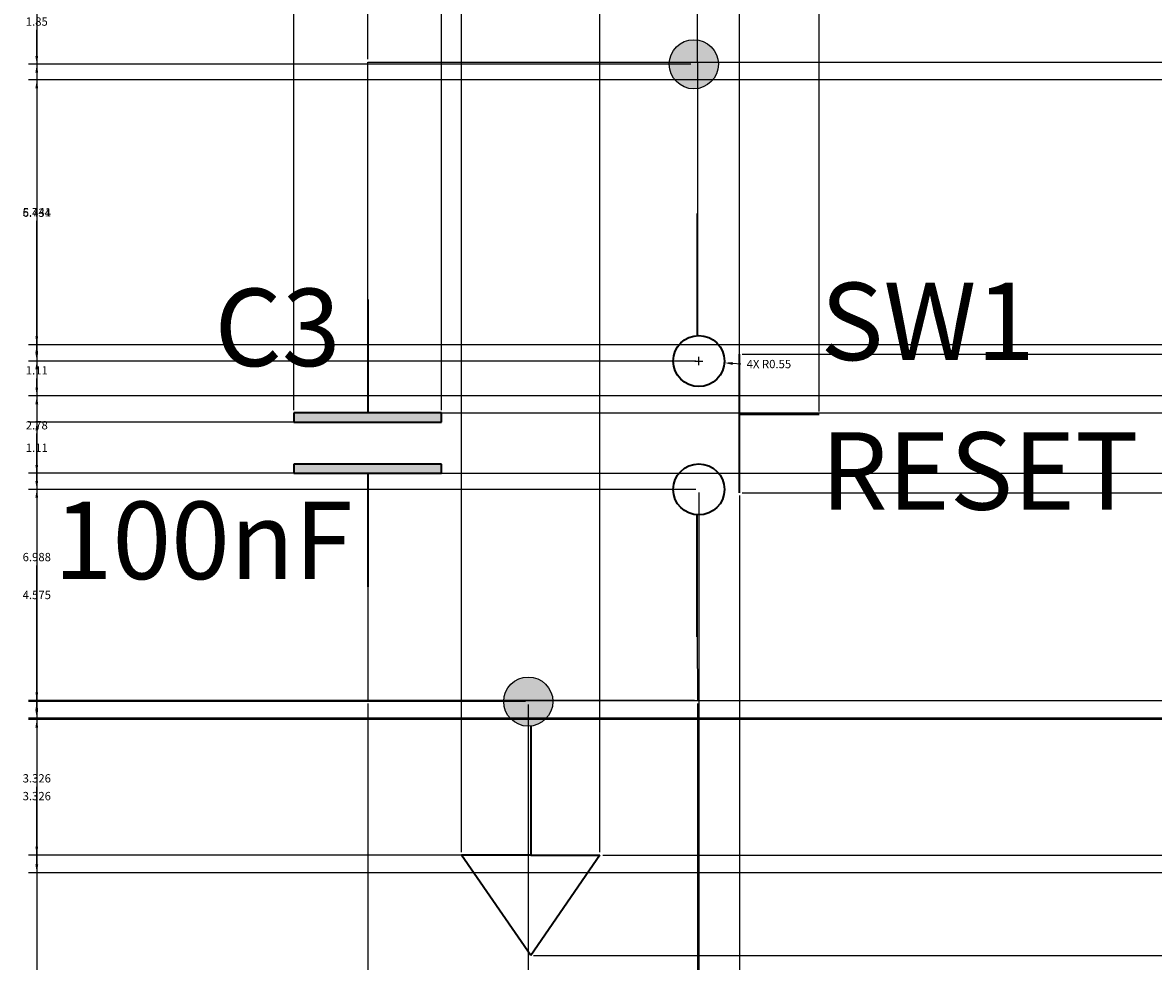
# Model space of a CAD drawing. Units: inches. Extents: x 23 to 132, y 5 to 105.
# Tile 2 of 14: x 23 to 47, y 54 to 75. Entities that reach past the tile are written whole.
import ezdxf

# ---------------------------------------------------------------- set-up
doc = ezdxf.new("R2010")
doc.units = ezdxf.units.IN
doc.header["$MEASUREMENT"] = 0
for name, color, linetype, lineweight in [('A-ANNO-DIMS', 2, 'Continuous', 18), ('E-ANNO-IDEN', 4, 'Continuous', 18), ('E-SYMB', 1, 'Continuous', 35), ('E-SYMB-PATT', 1, 'Continuous', 18), ('E-WIRE', 3, 'Continuous', 25), ('E-WIRE-PATT', 3, 'Continuous', 18)]:
    doc.layers.add(name, color=color, linetype=linetype, lineweight=lineweight)
doc.styles.get("Standard").update_dxf_attribs({"font": 'arial.ttf'})
doc.dimstyles.get("Standard").update_dxf_attribs({"dimtxt": 0.18, "dimasz": 0.18, "dimexe": 0.18, "dimexo": 0.0625, "dimgap": 0.09, "dimtad": 0, "dimtih": 1, "dimtoh": 1, "dimdec": 4, "dimzin": 0, "dimdsep": 46, "dimtxsty": 'Standard', "dimcen": 0.09, "dimadec": 0, "dimazin": 0, "dimtfac": 1, "dimtdec": 4, "dimtofl": 0, "dimtmove": 0, "dimatfit": 3, "dimfxl": 1, "dimtolj": 1, "dimtzin": 0, "dimarcsym": 0})

# ---------------------------------------------------------------- blocks, each defined once
blk = doc.blocks.new('GND')
for p, q in [((1.5, 4.977), (1.5, 2.181)), ((1.5, 2.181), (0, 2.181)), ((1.5, 0), (0, 2.181)), ((1.5, 2.181), (3, 2.181)), ((3, 2.181), (1.5, 0))]:
    blk.add_line(p, q)
blk = doc.blocks.new('*D2')
at = {"layer": 'A-ANNO-DIMS', "color": 0, "lineweight": -2, "transparency": 16777216}
for p, q in [((28.697, 66.272), (28.697, 105.232)), ((123.211, 99.539), (123.211, 105.232)), ((28.877, 105.052), (75.577, 105.052)), ((123.031, 105.052), (76.33, 105.052))]:
    blk.add_line(p, q, dxfattribs=at)
at = {"layer": 'A-ANNO-DIMS', "color": 0, "transparency": 16777216}
for points in [[(28.877, 105.082), (28.877, 105.022), (28.697, 105.052)], [(123.031, 105.082), (123.031, 105.022), (123.211, 105.052)]]:
    blk.add_solid(points, dxfattribs=at)
at = {"layer": 'Defpoints', "color": 0, "transparency": 16777216}
for p in [(123.211, 105.052), (123.211, 99.477), (28.697, 66.21)]:
    blk.add_point(p, dxfattribs=at)
at = {"layer": 'A-ANNO-DIMS', "color": 0, "transparency": 16777216, "insert": (75.954, 105.052), "char_height": 0.18, "attachment_point": 5}
blk.add_mtext('\\A1;94.51', dxfattribs=at)
blk = doc.blocks.new('*D6')
at = {"layer": 'A-ANNO-DIMS', "color": 0, "lineweight": -2, "transparency": 16777216}
for p, q in [((50.202, 77.095), (22.942, 77.095)), ((23.122, 76.915), (23.122, 47.733)), ((23.122, 18.187), (23.122, 47.369)), ((50.202, 18.007), (22.942, 18.007))]:
    blk.add_line(p, q, dxfattribs=at)
at = {"layer": 'A-ANNO-DIMS', "color": 0, "transparency": 16777216}
for points in [[(23.092, 76.915), (23.152, 76.915), (23.122, 77.095)], [(23.092, 18.187), (23.152, 18.187), (23.122, 18.007)]]:
    blk.add_solid(points, dxfattribs=at)
at = {"layer": 'Defpoints', "color": 0, "transparency": 16777216}
for p in [(23.122, 77.095), (50.265, 77.095), (50.265, 18.007)]:
    blk.add_point(p, dxfattribs=at)
at = {"layer": 'A-ANNO-DIMS', "color": 0, "transparency": 16777216, "insert": (23.122, 47.551), "char_height": 0.18, "attachment_point": 5}
blk.add_mtext('\\A1;59.09', dxfattribs=at)
blk = doc.blocks.new('*D7')
at = {"layer": 'A-ANNO-DIMS', "color": 0, "lineweight": -2, "transparency": 16777216}
for p, q in [((30.295, 73.877), (30.295, 105.232)), ((50.265, 77.157), (50.265, 105.232)), ((30.475, 105.052), (39.895, 105.052)), ((50.085, 105.052), (40.665, 105.052))]:
    blk.add_line(p, q, dxfattribs=at)
at = {"layer": 'A-ANNO-DIMS', "color": 0, "transparency": 16777216}
for points in [[(30.475, 105.082), (30.475, 105.022), (30.295, 105.052)], [(50.085, 105.082), (50.085, 105.022), (50.265, 105.052)]]:
    blk.add_solid(points, dxfattribs=at)
at = {"layer": 'Defpoints', "color": 0, "transparency": 16777216}
for p in [(50.265, 105.052), (50.265, 77.095), (30.295, 73.814)]:
    blk.add_point(p, dxfattribs=at)
at = {"layer": 'A-ANNO-DIMS', "color": 0, "transparency": 16777216, "insert": (40.28, 105.052), "char_height": 0.18, "attachment_point": 5}
blk.add_mtext('\\A1;19.97', dxfattribs=at)
blk = doc.blocks.new('*D55')
at = {"layer": 'A-ANNO-DIMS', "color": 0, "lineweight": -2, "transparency": 16777216}
for p, q in [((30.295, 59.913), (30.295, 5.443)), ((33.776, 59.889), (33.776, 5.443)), ((30.475, 5.623), (31.712, 5.623)), ((33.596, 5.623), (32.359, 5.623))]:
    blk.add_line(p, q, dxfattribs=at)
at = {"layer": 'A-ANNO-DIMS', "color": 0, "transparency": 16777216}
for points in [[(30.475, 5.653), (30.475, 5.593), (30.295, 5.623)], [(33.596, 5.653), (33.596, 5.593), (33.776, 5.623)]]:
    blk.add_solid(points, dxfattribs=at)
at = {"layer": 'Defpoints', "color": 0, "transparency": 16777216}
for p in [(30.295, 59.975), (33.776, 59.951), (33.776, 5.623)]:
    blk.add_point(p, dxfattribs=at)
at = {"layer": 'A-ANNO-DIMS', "color": 0, "transparency": 16777216, "insert": (32.036, 5.623), "char_height": 0.18, "attachment_point": 5}
blk.add_mtext('\\A1;3.48', dxfattribs=at)
blk = doc.blocks.new('*D56')
at = {"layer": 'A-ANNO-DIMS', "color": 0, "lineweight": -2, "transparency": 16777216}
for p, q in [((33.776, 59.889), (33.776, 5.443)), ((37.442, 59.913), (37.442, 5.443)), ((33.956, 5.623), (35.215, 5.623)), ((37.262, 5.623), (36.002, 5.623))]:
    blk.add_line(p, q, dxfattribs=at)
at = {"layer": 'A-ANNO-DIMS', "color": 0, "transparency": 16777216}
for points in [[(33.956, 5.653), (33.956, 5.593), (33.776, 5.623)], [(37.262, 5.653), (37.262, 5.593), (37.442, 5.623)]]:
    blk.add_solid(points, dxfattribs=at)
at = {"layer": 'Defpoints', "color": 0, "transparency": 16777216}
for p in [(33.776, 59.951), (37.442, 59.975), (37.442, 5.623)]:
    blk.add_point(p, dxfattribs=at)
at = {"layer": 'A-ANNO-DIMS', "color": 0, "transparency": 16777216, "insert": (35.609, 5.623), "char_height": 0.18, "attachment_point": 5}
blk.add_mtext('\\A1;3.666', dxfattribs=at)
blk = doc.blocks.new('*D57')
at = {"layer": 'A-ANNO-DIMS', "color": 0, "lineweight": -2, "transparency": 16777216}
for p, q in [((30.358, 64.901), (129.239, 64.901)), ((129.059, 64.721), (129.059, 62.62)), ((129.059, 60.155), (129.059, 62.256)), ((30.358, 59.975), (129.239, 59.975))]:
    blk.add_line(p, q, dxfattribs=at)
at = {"layer": 'A-ANNO-DIMS', "color": 0, "transparency": 16777216}
for points in [[(129.029, 64.721), (129.089, 64.721), (129.059, 64.901)], [(129.029, 60.155), (129.089, 60.155), (129.059, 59.975)]]:
    blk.add_solid(points, dxfattribs=at)
at = {"layer": 'Defpoints', "color": 0, "transparency": 16777216}
for p in [(30.295, 64.901), (129.059, 64.901), (30.295, 59.975)]:
    blk.add_point(p, dxfattribs=at)
at = {"layer": 'A-ANNO-DIMS', "color": 0, "transparency": 16777216, "insert": (129.059, 62.438), "char_height": 0.18, "attachment_point": 5}
blk.add_mtext('\\A1;4.925', dxfattribs=at)
blk = doc.blocks.new('*D58')
at = {"layer": 'A-ANNO-DIMS', "color": 0, "lineweight": -2, "transparency": 16777216}
for p, q in [((30.358, 73.814), (129.239, 73.814)), ((129.059, 73.634), (129.059, 70.194)), ((129.059, 66.39), (129.059, 69.83)), ((30.359, 66.21), (129.239, 66.21))]:
    blk.add_line(p, q, dxfattribs=at)
at = {"layer": 'A-ANNO-DIMS', "color": 0, "transparency": 16777216}
for points in [[(129.029, 73.634), (129.089, 73.634), (129.059, 73.814)], [(129.029, 66.39), (129.089, 66.39), (129.059, 66.21)]]:
    blk.add_solid(points, dxfattribs=at)
at = {"layer": 'Defpoints', "color": 0, "transparency": 16777216}
for p in [(30.295, 73.814), (129.059, 73.814), (30.297, 66.21)]:
    blk.add_point(p, dxfattribs=at)
at = {"layer": 'A-ANNO-DIMS', "color": 0, "transparency": 16777216, "insert": (129.059, 70.012), "char_height": 0.18, "attachment_point": 5}
blk.add_mtext('\\A1;7.604', dxfattribs=at)
blk = doc.blocks.new('*D59')
at = {"layer": 'A-ANNO-DIMS', "color": 0, "lineweight": -2, "transparency": 16777216}
for p, q in [((31.834, 66.01), (22.942, 66.01)), ((23.122, 65.83), (23.122, 65.636)), ((23.122, 65.081), (23.122, 65.275)), ((31.834, 64.901), (22.942, 64.901))]:
    blk.add_line(p, q, dxfattribs=at)
at = {"layer": 'A-ANNO-DIMS', "color": 0, "transparency": 16777216}
for points in [[(23.092, 65.83), (23.152, 65.83), (23.122, 66.01)], [(23.092, 65.081), (23.152, 65.081), (23.122, 64.901)]]:
    blk.add_solid(points, dxfattribs=at)
at = {"layer": 'Defpoints', "color": 0, "transparency": 16777216}
for p in [(23.122, 66.01), (31.897, 66.01), (31.897, 64.901)]:
    blk.add_point(p, dxfattribs=at)
at = {"layer": 'A-ANNO-DIMS', "color": 0, "transparency": 16777216, "insert": (23.122, 65.455), "char_height": 0.18, "attachment_point": 5}
blk.add_mtext('\\A1;1.11', dxfattribs=at)
blk = doc.blocks.new('*D60')
at = {"layer": 'A-ANNO-DIMS', "color": 0, "lineweight": -2, "transparency": 16777216}
for p, q in [((28.697, 66.272), (28.697, 105.232)), ((31.897, 66.272), (31.897, 105.232)), ((28.877, 105.052), (30.044, 105.052)), ((31.717, 105.052), (30.549, 105.052))]:
    blk.add_line(p, q, dxfattribs=at)
at = {"layer": 'A-ANNO-DIMS', "color": 0, "transparency": 16777216}
for points in [[(28.877, 105.082), (28.877, 105.022), (28.697, 105.052)], [(31.717, 105.082), (31.717, 105.022), (31.897, 105.052)]]:
    blk.add_solid(points, dxfattribs=at)
at = {"layer": 'Defpoints', "color": 0, "transparency": 16777216}
for p in [(31.897, 105.052), (28.697, 66.21), (31.897, 66.21)]:
    blk.add_point(p, dxfattribs=at)
at = {"layer": 'A-ANNO-DIMS', "color": 0, "transparency": 16777216, "insert": (30.297, 105.052), "char_height": 0.18, "attachment_point": 5}
blk.add_mtext('\\A1;3.2', dxfattribs=at)
blk = doc.blocks.new('*D61')
at = {"layer": 'A-ANNO-DIMS', "color": 0, "lineweight": -2, "transparency": 16777216}
for p, q in [((37.411, 64.551), (22.942, 64.551)), ((23.122, 64.371), (23.122, 62.445)), ((23.122, 60.155), (23.122, 62.081)), ((37.38, 59.975), (22.942, 59.975))]:
    blk.add_line(p, q, dxfattribs=at)
at = {"layer": 'A-ANNO-DIMS', "color": 0, "transparency": 16777216}
for points in [[(23.092, 64.371), (23.152, 64.371), (23.122, 64.551)], [(23.092, 60.155), (23.152, 60.155), (23.122, 59.975)]]:
    blk.add_solid(points, dxfattribs=at)
at = {"layer": 'Defpoints', "color": 0, "transparency": 16777216}
for p in [(23.122, 64.551), (37.473, 64.551), (37.442, 59.975)]:
    blk.add_point(p, dxfattribs=at)
at = {"layer": 'A-ANNO-DIMS', "color": 0, "transparency": 16777216, "insert": (23.122, 62.263), "char_height": 0.18, "attachment_point": 5}
blk.add_mtext('\\A1;4.575', dxfattribs=at)
blk = doc.blocks.new('*D62')
at = {"layer": 'A-ANNO-DIMS', "color": 0, "lineweight": -2, "transparency": 16777216}
for p, q in [((37.411, 67.334), (22.942, 67.334)), ((23.122, 67.154), (23.122, 66.124)), ((23.122, 64.731), (23.122, 65.76)), ((37.411, 64.551), (22.942, 64.551))]:
    blk.add_line(p, q, dxfattribs=at)
at = {"layer": 'A-ANNO-DIMS', "color": 0, "transparency": 16777216}
for points in [[(23.092, 67.154), (23.152, 67.154), (23.122, 67.334)], [(23.092, 64.731), (23.152, 64.731), (23.122, 64.551)]]:
    blk.add_solid(points, dxfattribs=at)
at = {"layer": 'Defpoints', "color": 0, "transparency": 16777216}
for p in [(23.122, 67.334), (37.473, 67.334), (37.473, 64.551)]:
    blk.add_point(p, dxfattribs=at)
at = {"layer": 'A-ANNO-DIMS', "color": 0, "transparency": 16777216, "insert": (23.122, 65.942), "char_height": 0.18, "attachment_point": 5}
blk.add_mtext('\\A1;2.78', dxfattribs=at)
blk = doc.blocks.new('*D63')
at = {"layer": 'A-ANNO-DIMS', "color": 0, "lineweight": -2, "transparency": 16777216}
for p, q in [((37.3, 73.768), (22.942, 73.768)), ((23.122, 73.588), (23.122, 70.733)), ((23.122, 67.514), (23.122, 70.369)), ((37.411, 67.334), (22.942, 67.334))]:
    blk.add_line(p, q, dxfattribs=at)
at = {"layer": 'A-ANNO-DIMS', "color": 0, "transparency": 16777216}
for points in [[(23.092, 73.588), (23.152, 73.588), (23.122, 73.768)], [(23.092, 67.514), (23.152, 67.514), (23.122, 67.334)]]:
    blk.add_solid(points, dxfattribs=at)
at = {"layer": 'Defpoints', "color": 0, "transparency": 16777216}
for p in [(23.122, 73.768), (37.363, 73.768), (37.473, 67.334)]:
    blk.add_point(p, dxfattribs=at)
at = {"layer": 'A-ANNO-DIMS', "color": 0, "transparency": 16777216, "insert": (23.122, 70.551), "char_height": 0.18, "attachment_point": 5}
blk.add_mtext('\\A1;6.434', dxfattribs=at)
blk = doc.blocks.new('*D64')
at = {"layer": 'A-ANNO-DIMS', "color": 0, "lineweight": -2, "transparency": 16777216}
for p, q in [((37.381, 75.621), (22.942, 75.621)), ((23.122, 75.441), (23.122, 74.876)), ((23.122, 73.948), (23.122, 74.513)), ((37.3, 73.768), (22.942, 73.768))]:
    blk.add_line(p, q, dxfattribs=at)
at = {"layer": 'A-ANNO-DIMS', "color": 0, "transparency": 16777216}
for points in [[(23.092, 75.441), (23.152, 75.441), (23.122, 75.621)], [(23.092, 73.948), (23.152, 73.948), (23.122, 73.768)]]:
    blk.add_solid(points, dxfattribs=at)
at = {"layer": 'Defpoints', "color": 0, "transparency": 16777216}
for p in [(23.122, 75.621), (37.443, 75.621), (37.363, 73.768)]:
    blk.add_point(p, dxfattribs=at)
at = {"layer": 'A-ANNO-DIMS', "color": 0, "transparency": 16777216, "insert": (23.122, 74.694), "char_height": 0.18, "attachment_point": 5}
blk.add_mtext('\\A1;1.85', dxfattribs=at)
blk = doc.blocks.new('*D65')
at = {"layer": 'A-ANNO-DIMS', "color": 0, "lineweight": -2, "transparency": 16777216}
for p, q in [((38.414, 67.485), (129.239, 67.485)), ((129.059, 67.305), (129.059, 66.165)), ((129.059, 64.66), (129.059, 65.801)), ((38.414, 64.48), (129.239, 64.48))]:
    blk.add_line(p, q, dxfattribs=at)
at = {"layer": 'A-ANNO-DIMS', "color": 0, "transparency": 16777216}
for points in [[(129.029, 67.305), (129.089, 67.305), (129.059, 67.485)], [(129.029, 64.66), (129.089, 64.66), (129.059, 64.48)]]:
    blk.add_solid(points, dxfattribs=at)
at = {"layer": 'Defpoints', "color": 0, "transparency": 16777216}
for p in [(38.351, 67.485), (129.059, 67.485), (38.351, 64.48)]:
    blk.add_point(p, dxfattribs=at)
at = {"layer": 'A-ANNO-DIMS', "color": 0, "transparency": 16777216, "insert": (129.059, 65.983), "char_height": 0.18, "attachment_point": 5}
blk.add_mtext('\\A1;3.005', dxfattribs=at)
blk = doc.blocks.new('*D66')
at = {"layer": 'A-ANNO-DIMS', "color": 0, "lineweight": -2, "transparency": 16777216}
for p, q in [((37.473, 64.488), (37.473, 5.443)), ((38.351, 64.418), (38.351, 5.443)), ((37.293, 5.623), (37.113, 5.623)), ((38.531, 5.623), (38.711, 5.623))]:
    blk.add_line(p, q, dxfattribs=at)
at = {"layer": 'A-ANNO-DIMS', "color": 0, "transparency": 16777216}
for points in [[(37.293, 5.653), (37.293, 5.593), (37.473, 5.623)], [(38.531, 5.653), (38.531, 5.593), (38.351, 5.623)]]:
    blk.add_solid(points, dxfattribs=at)
at = {"layer": 'Defpoints', "color": 0, "transparency": 16777216}
for p in [(37.473, 64.551), (38.351, 64.48), (38.351, 5.623)]:
    blk.add_point(p, dxfattribs=at)
at = {"layer": 'A-ANNO-DIMS', "color": 0, "transparency": 16777216, "insert": (37.912, 5.623), "char_height": 0.18, "attachment_point": 5}
blk.add_mtext('\\A1;0.88', dxfattribs=at)
blk = doc.blocks.new('*D67')
at = {"layer": 'A-ANNO-DIMS', "color": 0, "lineweight": -2, "transparency": 16777216}
for p, q in [((38.351, 66.244), (38.351, 105.232)), ((40.084, 66.244), (40.084, 105.232)), ((38.531, 105.052), (38.902, 105.052)), ((39.904, 105.052), (39.533, 105.052))]:
    blk.add_line(p, q, dxfattribs=at)
at = {"layer": 'A-ANNO-DIMS', "color": 0, "transparency": 16777216}
for points in [[(38.531, 105.082), (38.531, 105.022), (38.351, 105.052)], [(39.904, 105.082), (39.904, 105.022), (40.084, 105.052)]]:
    blk.add_solid(points, dxfattribs=at)
at = {"layer": 'Defpoints', "color": 0, "transparency": 16777216}
for p in [(40.084, 105.052), (38.351, 66.181), (40.084, 66.181)]:
    blk.add_point(p, dxfattribs=at)
at = {"layer": 'A-ANNO-DIMS', "color": 0, "transparency": 16777216, "insert": (39.217, 105.052), "char_height": 0.18, "attachment_point": 5}
blk.add_mtext('\\A1;1.73', dxfattribs=at)
blk = doc.blocks.new('*D68')
at = {"layer": 'A-ANNO-DIMS', "color": 0, "lineweight": -2, "transparency": 16777216}
for p, q in [((33.713, 59.951), (22.942, 59.951)), ((23.122, 59.771), (23.122, 58.47)), ((23.122, 56.805), (23.122, 58.106)), ((33.767, 56.625), (22.942, 56.625))]:
    blk.add_line(p, q, dxfattribs=at)
at = {"layer": 'A-ANNO-DIMS', "color": 0, "transparency": 16777216}
for points in [[(23.092, 59.771), (23.152, 59.771), (23.122, 59.951)], [(23.092, 56.805), (23.152, 56.805), (23.122, 56.625)]]:
    blk.add_solid(points, dxfattribs=at)
at = {"layer": 'Defpoints', "color": 0, "transparency": 16777216}
for p in [(23.122, 59.951), (33.776, 59.951), (33.83, 56.625)]:
    blk.add_point(p, dxfattribs=at)
at = {"layer": 'A-ANNO-DIMS', "color": 0, "transparency": 16777216, "insert": (23.122, 58.288), "char_height": 0.18, "attachment_point": 5}
blk.add_mtext('\\A1;3.326', dxfattribs=at)
blk = doc.blocks.new('*D69')
at = {"layer": 'A-ANNO-DIMS', "color": 0, "lineweight": -2, "transparency": 16777216}
for p, q in [((32.33, 56.687), (32.33, 105.232)), ((35.33, 56.687), (35.33, 105.232)), ((32.51, 105.052), (33.681, 105.052)), ((35.15, 105.052), (33.979, 105.052))]:
    blk.add_line(p, q, dxfattribs=at)
at = {"layer": 'A-ANNO-DIMS', "color": 0, "transparency": 16777216}
for points in [[(32.51, 105.082), (32.51, 105.022), (32.33, 105.052)], [(35.15, 105.082), (35.15, 105.022), (35.33, 105.052)]]:
    blk.add_solid(points, dxfattribs=at)
at = {"layer": 'Defpoints', "color": 0, "transparency": 16777216}
for p in [(35.33, 105.052), (32.33, 56.625), (35.33, 56.625)]:
    blk.add_point(p, dxfattribs=at)
at = {"layer": 'A-ANNO-DIMS', "color": 0, "transparency": 16777216, "insert": (33.83, 105.052), "char_height": 0.18, "attachment_point": 5}
blk.add_mtext('\\A1;3', dxfattribs=at)
blk = doc.blocks.new('*D70')
at = {"layer": 'A-ANNO-DIMS', "color": 0, "lineweight": -2, "transparency": 16777216}
for p, q in [((35.392, 56.625), (129.239, 56.625)), ((129.059, 56.445), (129.059, 55.716)), ((129.059, 54.624), (129.059, 55.352)), ((33.892, 54.444), (129.239, 54.444))]:
    blk.add_line(p, q, dxfattribs=at)
at = {"layer": 'A-ANNO-DIMS', "color": 0, "transparency": 16777216}
for points in [[(129.029, 56.445), (129.089, 56.445), (129.059, 56.625)], [(129.029, 54.624), (129.089, 54.624), (129.059, 54.444)]]:
    blk.add_solid(points, dxfattribs=at)
at = {"layer": 'Defpoints', "color": 0, "transparency": 16777216}
for p in [(35.33, 56.625), (33.83, 54.444), (129.059, 54.444)]:
    blk.add_point(p, dxfattribs=at)
at = {"layer": 'A-ANNO-DIMS', "color": 0, "transparency": 16777216, "insert": (129.059, 55.534), "char_height": 0.18, "attachment_point": 5}
blk.add_mtext('\\A1;2.18', dxfattribs=at)
blk = doc.blocks.new('*D78')
at = {"layer": 'A-ANNO-DIMS', "color": 0, "lineweight": -2, "transparency": 16777216}
for p, q in [((112.773, 67.688), (22.942, 67.688)), ((23.122, 67.508), (23.122, 67.314)), ((23.122, 66.759), (23.122, 66.953)), ((112.773, 66.579), (22.942, 66.579))]:
    blk.add_line(p, q, dxfattribs=at)
at = {"layer": 'A-ANNO-DIMS', "color": 0, "transparency": 16777216}
for points in [[(23.092, 67.508), (23.152, 67.508), (23.122, 67.688)], [(23.092, 66.759), (23.152, 66.759), (23.122, 66.579)]]:
    blk.add_solid(points, dxfattribs=at)
at = {"layer": 'Defpoints', "color": 0, "transparency": 16777216}
for p in [(23.122, 67.688), (112.835, 67.688), (112.835, 66.579)]:
    blk.add_point(p, dxfattribs=at)
at = {"layer": 'A-ANNO-DIMS', "color": 0, "transparency": 16777216, "insert": (23.122, 67.133), "char_height": 0.18, "attachment_point": 5}
blk.add_mtext('\\A1;1.11', dxfattribs=at)
blk = doc.blocks.new('*D79')
at = {"layer": 'A-ANNO-DIMS', "color": 0, "lineweight": -2, "transparency": 16777216}
for p, q in [((114.373, 66.579), (22.942, 66.579)), ((23.122, 66.399), (23.122, 63.267)), ((23.122, 59.77), (23.122, 62.903)), ((114.371, 59.59), (22.942, 59.59))]:
    blk.add_line(p, q, dxfattribs=at)
at = {"layer": 'A-ANNO-DIMS', "color": 0, "transparency": 16777216}
for points in [[(23.092, 66.399), (23.152, 66.399), (23.122, 66.579)], [(23.092, 59.77), (23.152, 59.77), (23.122, 59.59)]]:
    blk.add_solid(points, dxfattribs=at)
at = {"layer": 'Defpoints', "color": 0, "transparency": 16777216}
for p in [(23.122, 66.579), (114.435, 66.579), (114.434, 59.59)]:
    blk.add_point(p, dxfattribs=at)
at = {"layer": 'A-ANNO-DIMS', "color": 0, "transparency": 16777216, "insert": (23.122, 63.085), "char_height": 0.18, "attachment_point": 5}
blk.add_mtext('\\A1;6.988', dxfattribs=at)
blk = doc.blocks.new('*D80')
at = {"layer": 'A-ANNO-DIMS', "color": 0, "lineweight": -2, "transparency": 16777216}
for p, q in [((114.373, 73.429), (22.942, 73.429)), ((23.122, 73.249), (23.122, 70.741)), ((23.122, 67.868), (23.122, 70.377)), ((114.373, 67.688), (22.942, 67.688))]:
    blk.add_line(p, q, dxfattribs=at)
at = {"layer": 'A-ANNO-DIMS', "color": 0, "transparency": 16777216}
for points in [[(23.092, 73.249), (23.152, 73.249), (23.122, 73.429)], [(23.092, 67.868), (23.152, 67.868), (23.122, 67.688)]]:
    blk.add_solid(points, dxfattribs=at)
at = {"layer": 'Defpoints', "color": 0, "transparency": 16777216}
for p in [(23.122, 73.429), (114.435, 73.429), (114.435, 67.688)]:
    blk.add_point(p, dxfattribs=at)
at = {"layer": 'A-ANNO-DIMS', "color": 0, "transparency": 16777216, "insert": (23.122, 70.559), "char_height": 0.18, "attachment_point": 5}
blk.add_mtext('\\A1;5.741', dxfattribs=at)
blk = doc.blocks.new('*D81')
at = {"layer": 'A-ANNO-DIMS', "color": 0, "lineweight": -2, "transparency": 16777216}
for p, q in [((110.705, 59.566), (22.942, 59.566)), ((23.122, 59.386), (23.122, 58.085)), ((23.122, 56.42), (23.122, 57.721)), ((110.759, 56.24), (22.942, 56.24))]:
    blk.add_line(p, q, dxfattribs=at)
at = {"layer": 'A-ANNO-DIMS', "color": 0, "transparency": 16777216}
for points in [[(23.092, 59.386), (23.152, 59.386), (23.122, 59.566)], [(23.092, 56.42), (23.152, 56.42), (23.122, 56.24)]]:
    blk.add_solid(points, dxfattribs=at)
at = {"layer": 'Defpoints', "color": 0, "transparency": 16777216}
for p in [(23.122, 59.566), (110.768, 59.566), (110.822, 56.24)]:
    blk.add_point(p, dxfattribs=at)
at = {"layer": 'A-ANNO-DIMS', "color": 0, "transparency": 16777216, "insert": (23.122, 57.903), "char_height": 0.18, "attachment_point": 5}
blk.add_mtext('\\A1;3.326', dxfattribs=at)
blk = doc.blocks.new('*D96')
at = {"layer": 'A-ANNO-DIMS', "color": 0, "lineweight": -2, "transparency": 16777216}
for p, q in [((37.473, 67.244), (37.473, 67.424)), ((37.383, 67.334), (37.563, 67.334)), ((38.384, 67.269), (38.205, 67.282))]:
    blk.add_line(p, q, dxfattribs=at)
at = {"layer": 'A-ANNO-DIMS', "color": 0, "transparency": 16777216}
blk.add_solid([(38.207, 67.312), (38.203, 67.252), (38.025, 67.295)], dxfattribs=at)
at = {"layer": 'Defpoints', "color": 0, "transparency": 16777216}
for p in [(37.473, 67.334), (38.025, 67.295)]:
    blk.add_point(p, dxfattribs=at)
at = {"layer": 'A-ANNO-DIMS', "color": 0, "transparency": 16777216, "insert": (38.992, 67.269), "char_height": 0.18, "attachment_point": 5}
blk.add_mtext('\\A1;4X R0.55', dxfattribs=at)

msp = doc.modelspace()

# ---------------------------------------------------------------- hatches: boundary and pattern name
at = {"layer": 'E-SYMB-PATT'}
h = msp.add_hatch(color=256, dxfattribs=at)
h.dxf.hatch_style = 1
h.paths.add_polyline_path([(28.6965, 66.2099), (28.6965, 66.0099), (31.8965, 66.0099), (31.8965, 66.2099), (30.2965, 66.2099)])
h.paths.add_polyline_path([(31.8965, 64.9007), (31.8965, 65.1007), (30.2965, 65.1007), (28.6965, 65.1007), (28.6965, 64.9007)])
at = {"layer": 'E-WIRE-PATT'}
h = msp.add_hatch(color=256, dxfattribs=at)
h.dxf.hatch_style = 1
h.paths.add_polyline_path([(41.2522, 75.6207), (42.3136, 75.6207, 0.9167819)])
h.paths.add_polyline_path([(42.3156, 75.5745, 0.0216975), (42.3136, 75.6207), (41.2522, 75.6207, 0.0216975), (41.2502, 75.5745, 1)])
h.paths.add_polyline_path([(37.4432, 74.2949), (37.4432, 73.8144), (37.4432, 73.2415, 0.3706245), (37.8957, 73.7682, 0.3706245)])
h.paths.add_polyline_path([(37.4432, 74.2949, 0.4331755), (36.8323, 73.8144), (37.4432, 73.8144)])
h.paths.add_polyline_path([(37.4432, 73.8144), (36.8323, 73.8144, 0.0216975), (36.8302, 73.7682, 0.4591888), (37.4432, 73.2415)])
h = msp.add_hatch(color=256, dxfattribs=at)
h.dxf.hatch_style = 1
h.paths.add_polyline_path([(34.3085, 59.951, 0.011463), (34.3079, 59.9755), (33.2436, 59.9755, 0.011463), (33.243, 59.951, 1)])
h.paths.add_polyline_path([(33.2436, 59.9755), (34.3079, 59.9755, 0.9551697)])

# ---------------------------------------------------------------- linework, layer by layer
at = {"layer": 'E-SYMB'}
for p, q in [((37.4432, 67.8869), (37.4432, 70.5326)), ((30.2965, 68.6693), (30.2965, 66.2099)), ((38.3512, 64.4801), (38.3512, 67.4851)), ((30.2965, 66.2099), (28.6965, 66.2099)), ((28.6965, 66.2099), (28.6965, 66.0099)), ((31.8965, 66.2099), (30.2965, 66.2099)), ((31.8965, 66.0099), (31.8965, 66.2099)), ((38.3512, 66.1814), (40.0835, 66.1814)), ((28.6965, 66.0099), (31.8965, 66.0099)), ((30.2965, 65.1007), (28.6965, 65.1007)), ((28.6965, 65.1007), (28.6965, 64.9007)), ((31.8965, 65.1007), (30.2965, 65.1007)), ((31.8965, 64.9007), (31.8965, 65.1007)), ((28.6965, 64.9007), (31.8965, 64.9007)), ((30.2954, 64.9007), (30.2954, 62.4412)), ((37.4387, 61.3524), (37.4387, 63.998))]:
    msp.add_line(p, q, dxfattribs=at)
for centre in [(37.473, 67.3342), (37.473, 64.5505)]:
    msp.add_circle(centre, 0.5536, dxfattribs=at)
at = {"layer": 'E-WIRE'}
for p, q in [((37.4432, 73.8144), (37.4432, 75.6207)), ((30.2954, 73.8144), (37.4432, 73.8144)), ((30.2965, 68.6693), (30.2954, 73.8144)), ((37.4432, 73.8144), (37.4432, 70.5326)), ((37.4387, 63.5454), (37.4387, 61.3524)), ((30.2954, 62.4412), (30.2954, 59.9755)), ((37.4387, 61.3524), (37.442, 59.9755)), ((30.2954, 59.9755), (37.442, 59.9755))]:
    msp.add_line(p, q, dxfattribs=at)
for centre in [(37.363, 73.7682), (33.7757, 59.951)]:
    msp.add_circle(centre, 0.5327, dxfattribs=at)

# ---------------------------------------------------------------- block references
at = {"layer": 'E-SYMB'}
msp.add_blockref('GND', (32.33, 54.4441), dxfattribs=at)

# ---------------------------------------------------------------- texts
at = {"layer": 'E-ANNO-IDEN'}
for s, p in [('C3', (26.9734, 67.2242)), ('SW1', (40.111, 67.3537)), ('RESET', (40.111, 64.1108)), ('100nF', (23.4909, 62.6075))]:
    msp.add_text(s, height=1.67943, dxfattribs=at).set_placement(p)

# ---------------------------------------------------------------- dimensions: what is measured, and where the dimension line sits
at = {"layer": 'A-ANNO-DIMS'}
for base, p1, p2, override, picture, middle in [((123.2107, 105.052), (28.6965, 66.2099), (123.2107, 99.477), {"dimdec": 2, "dimlfac": 1, "dimrnd": 0, "dimzin": 0, "dimdsep": 46, "dimlunit": 2}, '*D2', (75.9536, 105.052)), ((31.8965, 105.052), (28.6965, 66.2099), (31.8965, 66.2099), {"dimdec": 1, "dimlfac": 1, "dimrnd": 0, "dimzin": 0, "dimdsep": 46, "dimlunit": 2}, '*D60', (30.2965, 105.052)), ((50.2646, 105.052), (30.2954, 73.8144), (50.2646, 77.095), {"dimdec": 2, "dimlfac": 1, "dimrnd": 0, "dimzin": 0, "dimdsep": 46, "dimlunit": 2}, '*D7', (40.28, 105.052)), ((35.3299, 105.052), (32.3299, 56.6249), (35.3299, 56.6249), {"dimdec": 0, "dimlfac": 1, "dimrnd": 0, "dimzin": 0, "dimdsep": 46, "dimlunit": 2}, '*D69', (33.8299, 105.052)), ((40.0835, 105.052), (38.3512, 66.1814), (40.0835, 66.1814), {"dimdec": 2, "dimlfac": 1, "dimrnd": 0, "dimzin": 0, "dimdsep": 46, "dimlunit": 2}, '*D67', (39.2174, 105.052)), ((38.3512, 5.6233), (37.473, 64.5505), (38.3512, 64.4801), {"dimdec": 2, "dimlfac": 1, "dimrnd": 0, "dimzin": 0, "dimdsep": 46, "dimlunit": 2}, '*D66', (37.9121, 5.6233)), ((33.7757, 5.6233), (30.2954, 59.9755), (33.7757, 59.951), {"dimdec": 2, "dimlfac": 1, "dimrnd": 0, "dimzin": 0, "dimdsep": 46, "dimlunit": 2}, '*D55', (32.0356, 5.6233)), ((37.442, 5.6233), (33.7757, 59.951), (37.442, 59.9755), {"dimdec": 3, "dimlfac": 1, "dimrnd": 0, "dimzin": 0, "dimdsep": 46, "dimlunit": 2}, '*D56', (35.6089, 5.6233))]:
    dim = msp.add_linear_dim(base=base, p1=p1, p2=p2, dimstyle='Standard', override=override, dxfattribs=at)
    dim.commit()
    dim.dimension.update_dxf_attribs({"geometry": picture, "text_midpoint": middle})
for base, p1, p2, override, picture, middle in [((23.1215, 77.095), (50.2646, 18.0066), (50.2646, 77.095), {"dimdec": 2, "dimlfac": 1, "dimrnd": 0, "dimzin": 0, "dimdsep": 46, "dimlunit": 2}, '*D6', (23.1215, 47.5508)), ((23.1215, 75.6207), (37.363, 73.7682), (37.4432, 75.6207), {"dimdec": 2, "dimlfac": 1, "dimrnd": 0, "dimzin": 0, "dimdsep": 46, "dimlunit": 2}, '*D64', (23.1215, 74.6945)), ((129.05891, 73.81438), (30.29652, 66.20989), (30.29537, 73.81438), {"dimdec": 3, "dimlfac": 1, "dimrnd": 0, "dimzin": 0, "dimdsep": 46, "dimlunit": 2}, '*D58', (129.05891, 70.01213)), ((23.1215, 73.7682), (37.473, 67.3342), (37.363, 73.7682), {"dimdec": 3, "dimlfac": 1, "dimrnd": 0, "dimzin": 0, "dimdsep": 46, "dimlunit": 2}, '*D63', (23.1215, 70.5512)), ((23.1215, 73.4293), (114.4351, 67.6881), (114.4351, 73.4293), {"dimdec": 3, "dimlfac": 1, "dimrnd": 0, "dimzin": 0, "dimdsep": 46, "dimlunit": 2}, '*D80', (23.1215, 70.5587)), ((23.1215, 67.6881), (112.8351, 66.5788), (112.8351, 67.6881), {"dimdec": 2, "dimlfac": 1, "dimrnd": 0, "dimzin": 0, "dimdsep": 46, "dimlunit": 2}, '*D78', (23.1215, 67.1334)), ((129.0589, 67.4851), (38.3512, 64.4801), (38.3512, 67.4851), {"dimdec": 3, "dimlfac": 1, "dimrnd": 0, "dimzin": 0, "dimdsep": 46, "dimlunit": 2}, '*D65', (129.0589, 65.9826)), ((23.1215, 67.3342), (37.473, 64.5505), (37.473, 67.3342), {"dimdec": 2, "dimlfac": 1, "dimrnd": 0, "dimzin": 0, "dimdsep": 46, "dimlunit": 2}, '*D62', (23.1215, 65.9424)), ((23.1215, 66.5788), (114.434, 59.5904), (114.4351, 66.5788), {"dimdec": 3, "dimlfac": 1, "dimrnd": 0, "dimzin": 0, "dimdsep": 46, "dimlunit": 2}, '*D79', (23.1215, 63.0846)), ((23.1215, 66.0099), (31.8965, 64.9007), (31.8965, 66.0099), {"dimdec": 2, "dimlfac": 1, "dimrnd": 0, "dimzin": 0, "dimdsep": 46, "dimlunit": 2}, '*D59', (23.1215, 65.4553)), ((129.0589, 64.9007), (30.2954, 59.9755), (30.2954, 64.9007), {"dimdec": 3, "dimlfac": 1, "dimrnd": 0, "dimzin": 0, "dimdsep": 46, "dimlunit": 2}, '*D57', (129.0589, 62.4381)), ((23.1215, 64.5505), (37.442, 59.9755), (37.473, 64.5505), {"dimdec": 3, "dimlfac": 1, "dimrnd": 0, "dimzin": 0, "dimdsep": 46, "dimlunit": 2}, '*D61', (23.1215, 62.263)), ((23.1215, 59.951), (33.8299, 56.6249), (33.7757, 59.951), {"dimdec": 3, "dimlfac": 1, "dimrnd": 0, "dimzin": 0, "dimdsep": 46, "dimlunit": 2}, '*D68', (23.1215, 58.288)), ((23.1215, 59.566), (110.8219, 56.2399), (110.7677, 59.566), {"dimdec": 3, "dimlfac": 1, "dimrnd": 0, "dimzin": 0, "dimdsep": 46, "dimlunit": 2}, '*D81', (23.1215, 57.9029)), ((129.0589, 54.4437), (35.3299, 56.6249), (33.8299, 54.4437), {"dimdec": 2, "dimlfac": 1, "dimrnd": 0, "dimzin": 0, "dimdsep": 46, "dimlunit": 2}, '*D70', (129.0589, 55.5343))]:
    dim = msp.add_linear_dim(base=base, p1=p1, p2=p2, angle=90, dimstyle='Standard', override=override, dxfattribs=at)
    dim.commit()
    dim.dimension.update_dxf_attribs({"geometry": picture, "text_midpoint": middle})
dim = msp.add_radius_dim(center=(37.473, 67.3342), mpoint=(38.0252, 67.2946), text='4X <>', dimstyle='Standard', override={"dimdec": 2, "dimlfac": 1, "dimrnd": 0, "dimzin": 0, "dimdsep": 46, "dimlunit": 2}, dxfattribs=at)
dim.commit()
dim.dimension.update_dxf_attribs({"geometry": '*D96', "text_midpoint": (38.9919, 67.2689)})

doc.saveas('drawing.dxf')
